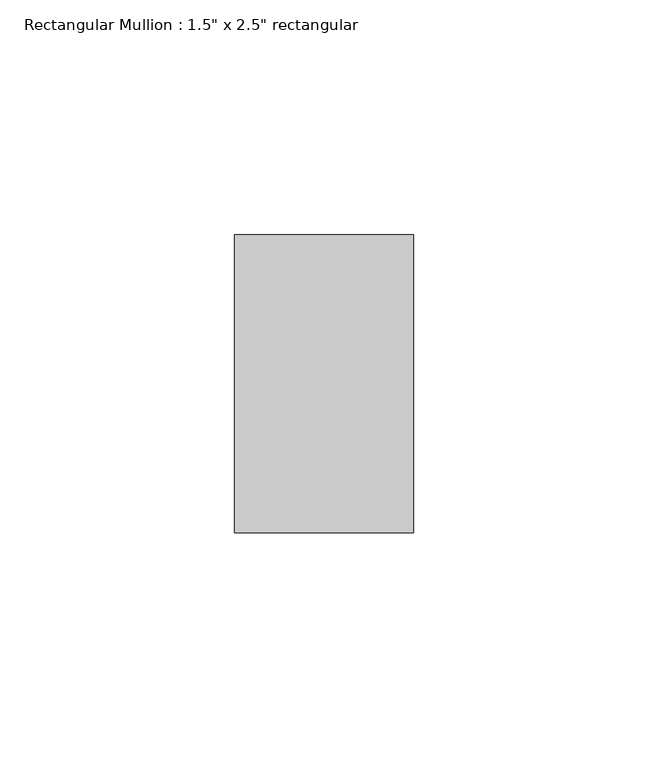
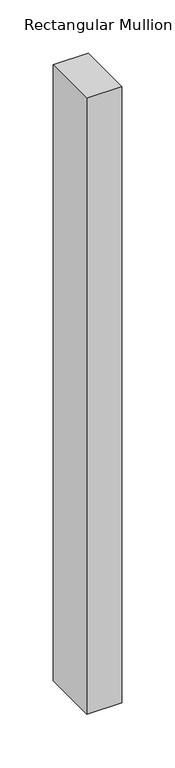
"""IFC4 building model written with IfcOpenShell, lengths in millimetres: member geometry."""

from ifc_helpers import new_model, si_unit, frame, origin, place, context, project, spatial, polyline, outline, extrude, source, transform, mapped, element, save


def member_594eddbe(model_context):
    return source(origin(), model_context, "Body", "SweptSolid", [
        extrude(outline(polyline([(0.0, 31.75), (0.0, -31.75), (-38.1, -31.75), (-38.1, 31.75), (0.0, 31.75)])), frame((0.0, 0.0, -709.1419508), z_axis=(0.0, 0.0, 1.0), x_axis=(1.0, 0.0, 0.0)), (0.0, 0.0, 1.0), 709.1419508),
    ])


if __name__ == "__main__":
    model = new_model("IFC4")
    model_context = context("Model", 3, world=origin())
    ifc_project = project(units=[si_unit("LENGTHUNIT", "METRE", prefix="MILLI")], contexts=[model_context])
    site = spatial("IfcSite", under=ifc_project)
    building = spatial("IfcBuilding", under=site)
    placement = place(None, origin())
    member_shape = member_594eddbe(model_context)
    element("IfcMember", 1, ObjectType="Rectangular Mullion : 1.5\" x 2.5\" rectangular", at=placement, inside=building, context=model_context, shape_type="MappedRepresentation", body=[
        mapped(member_shape, transform((0.0, 0.0, 0.0), x_axis=(1.0, 0.0, 0.0), y_axis=(0.0, 1.0, 0.0), z_axis=(0.0, 0.0, 1.0))),
    ])
    save(model, "model.ifc")

# Revit data of these elements
# Type "Rectangular Mullion : 1.5\" x 2.5\" rectangular"
#   built-in parameter 1007304 = 0.208333 (stored number, unit not read)
#   built-in parameter 1007301 = 0.0625 (stored number, unit not read)
#   built-in parameter 1007300 = 0.0625 (stored number, unit not read)
